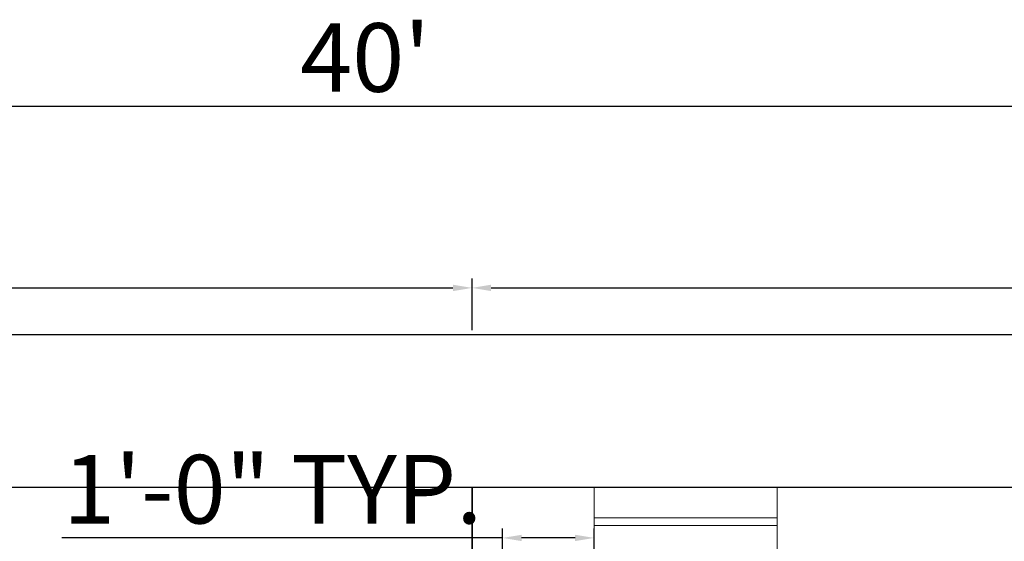
# Model space of a CAD drawing. Units: inches. Extents: x 3321 to 5237, y 11 to 1752.
# Tile 42 of 43: x 4881 to 5010, y 1680 to 1749. Entities that reach past the tile are written whole.
import ezdxf

# ---------------------------------------------------------------- set-up
doc = ezdxf.new("R2010")
doc.units = ezdxf.units.IN
for name, color, linetype, lineweight in [('A-ANNO-DIMS', 2, 'Continuous', 18), ('A-FLOR-EDGE', 7, 'Continuous', 25), ('A-GLAZ', 5, 'Continuous', 18), ('A-WALL', 7, 'Continuous', 35), ('C-PROP', 7, 'Continuous', 30)]:
    doc.layers.add(name, color=color, linetype=linetype, lineweight=lineweight)
doc.styles.get("Standard").update_dxf_attribs({"font": 'arial.ttf'})
doc.dimstyles.new('ISO-25', dxfattribs={"dimtxt": 9, "dimasz": 2.5, "dimexe": 1.25, "dimexo": 0.625, "dimtad": 1, "dimdec": 1, "dimlunit": 3, "dimtxsty": 'Standard', "dimcen": 2.5, "dimclrd": 4, "dimclre": 4, "dimclrt": 256, "dimadec": 0, "dimazin": 0, "dimtfac": 1, "dimtdec": 1, "dimtmove": 0, "dimatfit": 3, "dimfxl": 1, "dimarcsym": 0})

# ---------------------------------------------------------------- blocks, each defined once
blk = doc.blocks.new('*D13')
at = {"layer": 'A-ANNO-DIMS', "color": 0, "lineweight": -2, "transparency": 16777216}
for p, q in [((4731.08, 1707.96), (4731.08, 1714.75)), ((4940.08, 1707.96), (4940.08, 1714.75)), ((4733.58, 1713.5), (4937.58, 1713.5))]:
    blk.add_line(p, q, dxfattribs=at)
at = {"layer": 'A-ANNO-DIMS', "color": 0, "transparency": 16777216}
for points in [[(4733.58, 1713.92), (4733.58, 1713.08), (4731.08, 1713.5)], [(4937.58, 1713.92), (4937.58, 1713.08), (4940.08, 1713.5)]]:
    blk.add_solid(points, dxfattribs=at)
at = {"layer": 'Defpoints', "color": 0, "transparency": 16777216}
for p in [(4940.08, 1713.5), (4731.08, 1707.34), (4940.08, 1707.34)]:
    blk.add_point(p, dxfattribs=at)
at = {"layer": 'A-ANNO-DIMS', "color": 0, "transparency": 16777216, "insert": (4835.58, 1718.72), "char_height": 9, "attachment_point": 5}
blk.add_mtext('17\'-5"', dxfattribs=at)
blk = doc.blocks.new('*D14')
at = {"layer": 'A-ANNO-DIMS', "color": 0, "lineweight": -2, "transparency": 16777216}
for p, q in [((4940.08, 1707.96), (4940.08, 1714.75)), ((5130.08, 1707.96), (5130.08, 1714.75)), ((4942.58, 1713.5), (5127.58, 1713.5))]:
    blk.add_line(p, q, dxfattribs=at)
at = {"layer": 'A-ANNO-DIMS', "color": 0, "transparency": 16777216}
for points in [[(4942.58, 1713.92), (4942.58, 1713.08), (4940.08, 1713.5)], [(5127.58, 1713.92), (5127.58, 1713.08), (5130.08, 1713.5)]]:
    blk.add_solid(points, dxfattribs=at)
at = {"layer": 'Defpoints', "color": 0, "transparency": 16777216}
for p in [(5130.08, 1713.5), (4940.08, 1707.34), (5130.08, 1707.34)]:
    blk.add_point(p, dxfattribs=at)
at = {"layer": 'A-ANNO-DIMS', "color": 0, "transparency": 16777216, "insert": (5035.08, 1718.72), "char_height": 9, "attachment_point": 5}
blk.add_mtext('15\'-10"', dxfattribs=at)
blk = doc.blocks.new('*D149')
at = {"layer": 'A-ANNO-DIMS', "color": 0, "lineweight": -2, "transparency": 16777216}
for p, q in [((4686.08, 1707.96), (4686.08, 1738.58)), ((5166.08, 1707.96), (5166.08, 1738.58)), ((4688.58, 1737.33), (5163.58, 1737.33))]:
    blk.add_line(p, q, dxfattribs=at)
at = {"layer": 'A-ANNO-DIMS', "color": 0, "transparency": 16777216}
for points in [[(4688.58, 1737.74), (4688.58, 1736.91), (4686.08, 1737.33)], [(5163.58, 1737.74), (5163.58, 1736.91), (5166.08, 1737.33)]]:
    blk.add_solid(points, dxfattribs=at)
at = {"layer": 'Defpoints', "color": 0, "transparency": 16777216}
for p in [(5166.08, 1737.33), (4686.08, 1707.34), (5166.08, 1707.34)]:
    blk.add_point(p, dxfattribs=at)
at = {"layer": 'A-ANNO-DIMS', "color": 0, "transparency": 16777216, "insert": (4926.08, 1742.55), "char_height": 9, "attachment_point": 5}
blk.add_mtext("40'", dxfattribs=at)
blk = doc.blocks.new('WIN-24IN-9IN-WALL')
for p, q in [((9, 24), (0, 24)), ((4, 24), (4, 0)), ((5, 24), (5, 0)), ((9, 0), (0, 0))]:
    blk.add_line(p, q)
blk = doc.blocks.new('PROPERTY-40X60FT')
blk.add_line((0, 0), (480, 0))
blk = doc.blocks.new('*D202')
at = {"layer": 'A-ANNO-DIMS', "color": 4, "lineweight": -2, "transparency": 16777216}
for p, q in [((4944.08, 1678.96), (4944.08, 1681.96)), ((4956.09, 1678.96), (4956.09, 1681.96)), ((4944.08, 1680.71), (4886.32, 1680.71)), ((4953.59, 1680.71), (4946.58, 1680.71))]:
    blk.add_line(p, q, dxfattribs=at)
at = {"layer": 'A-ANNO-DIMS', "color": 4, "transparency": 16777216}
for points in [[(4946.58, 1681.12), (4946.58, 1680.29), (4944.08, 1680.71)], [(4953.59, 1681.12), (4953.59, 1680.29), (4956.09, 1680.71)]]:
    blk.add_solid(points, dxfattribs=at)
at = {"layer": 'Defpoints', "color": 0, "transparency": 16777216}
for p in [(4944.08, 1680.71), (4944.08, 1678.34), (4956.09, 1678.34)]:
    blk.add_point(p, dxfattribs=at)
at = {"layer": 'A-ANNO-DIMS', "transparency": 16777216, "insert": (4913.95, 1685.93), "char_height": 9, "attachment_point": 5}
blk.add_mtext('1\'-0" TYP.', dxfattribs=at)

msp = doc.modelspace()

# ---------------------------------------------------------------- linework, layer by layer
at = {"layer": 'A-FLOR-EDGE'}
msp.add_line((5130.08, 1687.34), (4731.08, 1687.34), dxfattribs=at)
at = {"layer": 'A-WALL'}
msp.add_line((4940.08, 1687.34), (4940.08, 1425.34), dxfattribs=at)

# ---------------------------------------------------------------- block references
at = {"layer": 'A-GLAZ', "rotation": 269.9999999999957}
msp.add_blockref('WIN-24IN-9IN-WALL', (4956.08, 1687.34), dxfattribs=at)
at = {"layer": 'C-PROP', "rotation": 180}
msp.add_blockref('PROPERTY-40X60FT', (5166.08, 1707.34), dxfattribs=at)

# ---------------------------------------------------------------- dimensions: what is measured, and where the dimension line sits
at = {"layer": 'A-ANNO-DIMS'}
for base, p1, p2, picture, middle in [((5166.08, 1737.33), (4686.08, 1707.34), (5166.08, 1707.34), '*D149', (4926.08, 1742.55)), ((4940.08, 1713.5), (4731.08, 1707.34), (4940.08, 1707.34), '*D13', (4835.58, 1718.72)), ((5130.08, 1713.5), (4940.08, 1707.34), (5130.08, 1707.34), '*D14', (5035.08, 1718.72))]:
    dim = msp.add_linear_dim(base=base, p1=p1, p2=p2, dimstyle='ISO-25', override={"dimclrd": 0, "dimclre": 0, "dimclrt": 0}, dxfattribs=at)
    dim.commit()
    dim.dimension.update_dxf_attribs({"geometry": picture, "text_midpoint": middle})
dim = msp.add_linear_dim(base=(4944.08, 1680.71), p1=(4956.09, 1678.34), p2=(4944.08, 1678.34), angle=180, text='<> TYP.', dimstyle='ISO-25', override={"dimdec": 1, "dimlfac": 1, "dimrnd": 0, "dimzin": 1, "dimdsep": 46, "dimlunit": 4, "dimfrac": 2}, dxfattribs=at)
dim.commit()
dim.dimension.update_dxf_attribs({"geometry": '*D202', "text_midpoint": (4913.95, 1685.93)})

doc.saveas('drawing.dxf')
